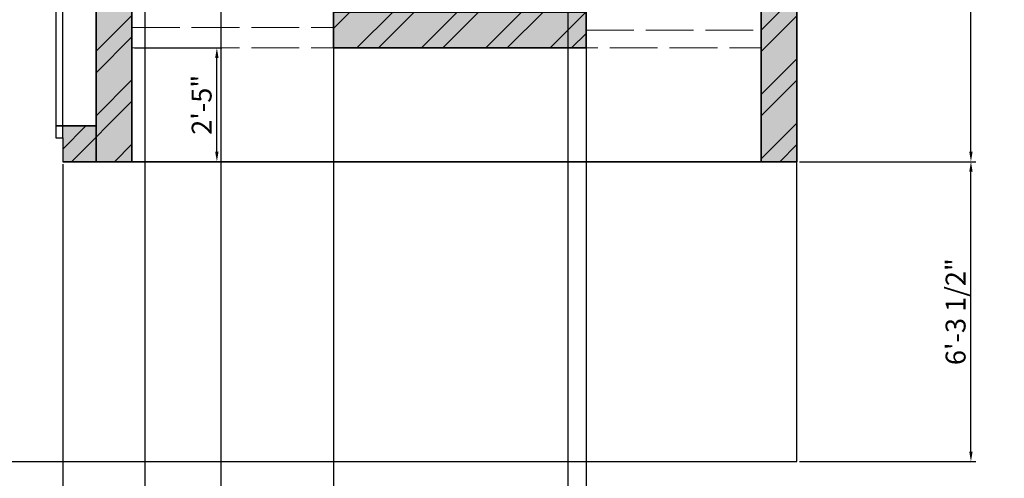
# Model space of a CAD drawing. Units: inches. Extents: x 1804 to 3296, y 909 to 2477.
# Tile 6 of 31: x 2130 to 2378, y 1059 to 1174. Entities that reach past the tile are written whole.
import ezdxf

# ---------------------------------------------------------------- set-up
doc = ezdxf.new("R2010")
doc.units = ezdxf.units.IN
doc.linetypes.add('ACAD_ISO02W100', pattern=[15, 12, -3])
for name, color, linetype, lineweight in [('A-ANNO-DIMS', 2, 'Continuous', 18), ('A-ANNO-TTLB', 156, 'Continuous', 35), ('A-GLAZ-OVHD', 130, 'ACAD_ISO02W100', 18), ('A-WALL-PATT', 10, 'Continuous', 13), ('C-PROP', 7, 'Continuous', 25), ('DOOR', 30, 'Continuous', 25), ('WALL', 10, 'Continuous', 35)]:
    doc.layers.add(name, color=color, linetype=linetype, lineweight=lineweight)
doc.styles.get("Standard").update_dxf_attribs({"font": 'arial.ttf'})
doc.dimstyles.new('ISO-25', dxfattribs={"dimtxt": 5, "dimasz": 2.5, "dimexe": 1.25, "dimexo": 0.625, "dimtad": 1, "dimdec": 0, "dimlunit": 4, "dimtxsty": 'Standard', "dimcen": 2.5, "dimadec": 0, "dimazin": 0, "dimtfac": 1, "dimtdec": 0, "dimtmove": 0, "dimatfit": 3, "dimfxl": 1, "dimarcsym": 0})

# ---------------------------------------------------------------- blocks, each defined once
blk = doc.blocks.new('*U2')
for p, q in [((0, 0), (0, -6)), ((40, 0), (40, -6))]:
    blk.add_line(p, q)
blk.add_lwpolyline([(0, 0), (0, 40), (1.75, 40), (1.75, 0)], close=True)
blk.add_arc((0, 0), 40, 0, 90)
blk = doc.blocks.new('*D20')
at = {"layer": 'A-ANNO-DIMS', "color": 0, "lineweight": -2, "transparency": 16777216}
for p, q in [((2159.2, 1166.63), (2181.16, 1166.63)), ((2179.91, 1140.57), (2179.91, 1164.13)), ((2159.2, 1138.07), (2181.16, 1138.07))]:
    blk.add_line(p, q, dxfattribs=at)
at = {"layer": 'A-ANNO-DIMS', "color": 0, "lineweight": 100, "transparency": 16777216}
for points in [[(2179.49, 1164.13), (2180.33, 1164.13), (2179.91, 1166.63)], [(2179.49, 1140.57), (2180.33, 1140.57), (2179.91, 1138.07)]]:
    blk.add_solid(points, dxfattribs=at)
at = {"layer": 'Defpoints', "color": 0, "lineweight": 100, "transparency": 16777216}
for p in [(2158.58, 1166.63), (2179.91, 1166.63), (2158.58, 1138.07)]:
    blk.add_point(p, dxfattribs=at)
at = {"layer": 'A-ANNO-DIMS', "color": 0, "transparency": 16777216, "insert": (2176.73, 1152.35), "char_height": 5, "attachment_point": 5, "rotation": 90}
blk.add_mtext('2\'-5"', dxfattribs=at)
blk = doc.blocks.new('*D22')
at = {"layer": 'A-ANNO-DIMS', "color": 0, "lineweight": -2, "transparency": 16777216}
for p, q in [((1934.58, 1147.69), (1934.58, 1206.88)), ((2149.58, 1147.69), (2149.58, 1206.88)), ((1937.08, 1205.63), (2147.08, 1205.63))]:
    blk.add_line(p, q, dxfattribs=at)
at = {"layer": 'A-ANNO-DIMS', "color": 0, "lineweight": 100, "transparency": 16777216}
for points in [[(1937.08, 1206.05), (1937.08, 1205.22), (1934.58, 1205.63)], [(2147.08, 1206.05), (2147.08, 1205.22), (2149.58, 1205.63)]]:
    blk.add_solid(points, dxfattribs=at)
at = {"layer": 'Defpoints', "color": 0, "lineweight": 100, "transparency": 16777216}
for p in [(2149.58, 1205.63), (1934.58, 1147.07), (2149.58, 1147.07)]:
    blk.add_point(p, dxfattribs=at)
at = {"layer": 'A-ANNO-DIMS', "color": 0, "transparency": 16777216, "insert": (2042.08, 1208.77), "char_height": 5, "attachment_point": 5}
blk.add_mtext('17\'-11"', dxfattribs=at)
blk = doc.blocks.new('*D53')
at = {"layer": 'A-ANNO-DIMS', "color": 0, "lineweight": -2, "transparency": 16777216}
for p, q in [((2326.16, 1793.38), (2370.49, 1793.38)), ((2369.24, 1140.57), (2369.24, 1790.88)), ((2326.16, 1138.07), (2370.49, 1138.07))]:
    blk.add_line(p, q, dxfattribs=at)
at = {"layer": 'A-ANNO-DIMS', "color": 0, "lineweight": 100, "transparency": 16777216}
for points in [[(2368.82, 1790.88), (2369.65, 1790.88), (2369.24, 1793.38)], [(2368.82, 1140.57), (2369.65, 1140.57), (2369.24, 1138.07)]]:
    blk.add_solid(points, dxfattribs=at)
at = {"layer": 'Defpoints', "color": 0, "lineweight": 100, "transparency": 16777216}
for p in [(2325.54, 1793.38), (2369.24, 1793.38), (2325.54, 1138.07)]:
    blk.add_point(p, dxfattribs=at)
at = {"layer": 'A-ANNO-DIMS', "color": 0, "transparency": 16777216, "insert": (2366.03, 1465.72), "char_height": 5, "attachment_point": 5, "rotation": 90}
blk.add_mtext('54\'-7 1/2"', dxfattribs=at)
blk = doc.blocks.new('*D54')
at = {"layer": 'A-ANNO-DIMS', "color": 0, "lineweight": -2, "transparency": 16777216}
for p, q in [((2326.16, 1138.07), (2370.49, 1138.07)), ((2369.24, 1065.27), (2369.24, 1135.57)), ((2326.16, 1062.77), (2370.49, 1062.77))]:
    blk.add_line(p, q, dxfattribs=at)
at = {"layer": 'A-ANNO-DIMS', "color": 0, "lineweight": 100, "transparency": 16777216}
for points in [[(2368.82, 1135.57), (2369.65, 1135.57), (2369.24, 1138.07)], [(2368.82, 1065.27), (2369.65, 1065.27), (2369.24, 1062.77)]]:
    blk.add_solid(points, dxfattribs=at)
at = {"layer": 'Defpoints', "color": 0, "lineweight": 100, "transparency": 16777216}
for p in [(2325.54, 1138.07), (2369.24, 1138.07), (2325.54, 1062.77)]:
    blk.add_point(p, dxfattribs=at)
at = {"layer": 'A-ANNO-DIMS', "color": 0, "transparency": 16777216, "insert": (2366.03, 1100.42), "char_height": 5, "attachment_point": 5, "rotation": 90}
blk.add_mtext('6\'-3 1/2"', dxfattribs=at)
blk = doc.blocks.new('*D56')
at = {"layer": 'A-ANNO-DIMS', "color": 0, "lineweight": -2, "transparency": 16777216}
for p, q in [((2180.87, 1680.42), (2180.87, 975.89)), ((2268, 1680.42), (2268, 975.89)), ((2183.37, 977.14), (2265.5, 977.14))]:
    blk.add_line(p, q, dxfattribs=at)
at = {"layer": 'A-ANNO-DIMS', "color": 0, "lineweight": 100, "transparency": 16777216}
for points in [[(2183.37, 977.56), (2183.37, 976.72), (2180.87, 977.14)], [(2265.5, 977.56), (2265.5, 976.72), (2268, 977.14)]]:
    blk.add_solid(points, dxfattribs=at)
at = {"layer": 'Defpoints', "color": 0, "lineweight": 100, "transparency": 16777216}
for p in [(2180.87, 1681.04), (2268, 1681.04), (2268, 977.14)]:
    blk.add_point(p, dxfattribs=at)
at = {"layer": 'A-ANNO-DIMS', "color": 0, "transparency": 16777216, "insert": (2224.44, 980.32), "char_height": 5, "attachment_point": 5}
blk.add_mtext('7\'-3"', dxfattribs=at)
blk = doc.blocks.new('*D59')
at = {"layer": 'A-ANNO-DIMS', "color": 0, "lineweight": -2, "transparency": 16777216}
for p, q in [((2121.83, 1590.3), (2121.83, 975.89)), ((2161.83, 1590.3), (2161.83, 975.89)), ((2124.33, 977.14), (2159.33, 977.14))]:
    blk.add_line(p, q, dxfattribs=at)
at = {"layer": 'A-ANNO-DIMS', "color": 0, "lineweight": 100, "transparency": 16777216}
for points in [[(2124.33, 977.56), (2124.33, 976.72), (2121.83, 977.14)], [(2159.33, 977.56), (2159.33, 976.72), (2161.83, 977.14)]]:
    blk.add_solid(points, dxfattribs=at)
at = {"layer": 'Defpoints', "color": 0, "lineweight": 100, "transparency": 16777216}
for p in [(2121.83, 1590.92), (2161.83, 1590.92), (2161.83, 977.14)]:
    blk.add_point(p, dxfattribs=at)
at = {"layer": 'A-ANNO-DIMS', "color": 0, "transparency": 16777216, "insert": (2141.83, 980.32), "char_height": 5, "attachment_point": 5}
blk.add_mtext('3\'-4"', dxfattribs=at)
blk = doc.blocks.new('*D61')
at = {"layer": 'A-ANNO-DIMS', "color": 0, "lineweight": -2, "transparency": 16777216}
for p, q in [((2101.21, 1137.44), (2101.21, 975.89)), ((2141.21, 1137.44), (2141.21, 975.89)), ((2103.71, 977.14), (2138.71, 977.14))]:
    blk.add_line(p, q, dxfattribs=at)
at = {"layer": 'A-ANNO-DIMS', "color": 0, "lineweight": 100, "transparency": 16777216}
for points in [[(2103.71, 977.56), (2103.71, 976.72), (2101.21, 977.14)], [(2138.71, 977.56), (2138.71, 976.72), (2141.21, 977.14)]]:
    blk.add_solid(points, dxfattribs=at)
at = {"layer": 'Defpoints', "color": 0, "lineweight": 100, "transparency": 16777216}
for p in [(2101.21, 1138.07), (2141.21, 1138.07), (2141.21, 977.14)]:
    blk.add_point(p, dxfattribs=at)
at = {"layer": 'A-ANNO-DIMS', "color": 0, "transparency": 16777216, "insert": (2121.21, 980.32), "char_height": 5, "attachment_point": 5}
blk.add_mtext('3\'-4"', dxfattribs=at)
blk = doc.blocks.new('*D69')
at = {"layer": 'A-ANNO-DIMS', "color": 0, "lineweight": -2, "transparency": 16777216}
for p, q in [((2209.19, 1223.01), (2209.19, 975.89)), ((2272.59, 1223.01), (2272.59, 975.89)), ((2211.69, 977.14), (2270.09, 977.14))]:
    blk.add_line(p, q, dxfattribs=at)
at = {"layer": 'A-ANNO-DIMS', "color": 0, "lineweight": 100, "transparency": 16777216}
for points in [[(2211.69, 977.56), (2211.69, 976.72), (2209.19, 977.14)], [(2270.09, 977.56), (2270.09, 976.72), (2272.59, 977.14)]]:
    blk.add_solid(points, dxfattribs=at)
at = {"layer": 'Defpoints', "color": 0, "lineweight": 100, "transparency": 16777216}
for p in [(2209.19, 1223.63), (2272.59, 1223.63), (2272.59, 977.14)]:
    blk.add_point(p, dxfattribs=at)
at = {"layer": 'A-ANNO-DIMS', "color": 0, "transparency": 16777216, "insert": (2240.89, 980.35), "char_height": 5, "attachment_point": 5}
blk.add_mtext('5\'-3 1/2"', dxfattribs=at)

msp = doc.modelspace()

# ---------------------------------------------------------------- hatches: boundary and pattern name
at = {"layer": 'A-ANNO-TTLB'}
h = msp.add_hatch(color=256, dxfattribs=at)
h.dxf.hatch_style = 1
h.paths.add_polyline_path([(3294.53, 2476.54), (1803.79, 2476.54), (1805.43, 909.47), (3296.17, 909.47)])
h.paths.add_polyline_path([(1811, 914.33), (1812.79, 2467.54), (3285.53, 2467.54), (3283.74, 914.33)], flags=16)
h.paths.add_polyline_path([(1925.58, 1062.77), (1925.58, 1138.07), (1925.58, 1539.88), (1925.58, 1793.38), (1925.58, 1830.04), (2325.54, 1830.04), (2325.54, 1793.38), (2325.54, 1586.42), (2325.54, 1138.07), (2325.54, 1062.77)], flags=0)
h.paths.add_polyline_path([(1997.22, 1029.4), (2008.85, 1037.96), (2008.85, 1020.84)], flags=0)
h.paths.add_polyline_path([(1934.58, 1138.07), (1934.58, 1147.07), (2078.77, 1147.07), (2078.77, 1138.07), (2060.94, 1138.07)], flags=0)
h.paths.add_polyline_path([(1944.35, 1138.07), (1944.35, 1147.07), (2056.05, 1147.07), (2056.05, 1138.07)], flags=0)
h.paths.add_polyline_path([(2222.24, 1037.96), (2233.87, 1029.4), (2222.24, 1020.84)], flags=0)
h.paths.add_polyline_path([(2061.94, 1139.07), (2061.94, 1146.07), (2077.77, 1146.07), (2077.77, 1139.07)], flags=0)
h.paths.add_polyline_path([(2149.58, 1138.07), (2149.58, 1269.44), (2158.58, 1269.44), (2158.58, 1326.69), (2149.58, 1326.69), (2149.58, 1340.94), (2139.6, 1340.94), (2139.6, 1434.25), (2149.58, 1434.25), (2149.58, 1447.36), (2158.58, 1447.36), (2158.58, 1423.87), (2158.58, 1408.06), (2198.46, 1408.06), (2198.46, 1412.56), (2282.65, 1412.56), (2282.65, 1465.94), (2316.54, 1465.94), (2316.54, 1590.92), (2192.86, 1590.92), (2192.86, 1595.3), (2291.17, 1595.3), (2291.17, 1590.92), (2316.54, 1590.92), (2316.54, 1784.38), (2300.24, 1784.38), (2300.24, 1757.47), (2268, 1757.47), (2268, 1681.04), (2180.87, 1681.04), (2180.87, 1757.47), (2148.63, 1757.47), (2148.63, 1784.38), (2119.08, 1784.38), (2119.08, 1585.58), (2114.58, 1585.58), (2114.58, 1784.38), (2064.11, 1784.38), (2046.28, 1784.38), (2046.28, 1760.38), (1958.58, 1760.38), (1958.58, 1664.38), (1934.58, 1664.38), (1934.58, 1784.38), (1934.58, 1793.38), (2046.28, 1793.38), (2064.11, 1793.38), (2119.08, 1793.38), (2230.78, 1793.38), (2230.78, 1784.38), (2268, 1784.38), (2300.24, 1784.38), (2316.54, 1784.38), (2316.54, 1590.92), (2316.54, 1373.73), (2316.54, 1138.07)], flags=0)
h.paths.add_polyline_path([(2209.19, 1166.63), (2209.19, 1175.63), (2158.58, 1175.63), (2209.19, 1223.63), (2209.19, 1231.63), (2183.88, 1231.63), (2183.88, 1301.66), (2242.59, 1301.66), (2242.59, 1326.69), (2316.54, 1326.69), (2272.59, 1271.63), (2272.59, 1223.63), (2316.54, 1175.63), (2272.59, 1175.63), (2272.59, 1166.63)], flags=0)
h.paths.add_polyline_path([(1947.77, 1345.22), (1947.77, 1457.48), (1991.2, 1457.48), (1991.2, 1451.7), (1991.2, 1352.18), (1991.2, 1345.22)], flags=0)
h.paths.add_polyline_path([(2209.19, 1271.63), (2262.59, 1271.63), (2262.59, 1311.85), (2272.59, 1301.66), (2272.59, 1271.63), (2269.92, 1269.63), (2270.59, 1269.63), (2270.59, 1225.63), (2211.19, 1225.63), (2211.19, 1269.63), (2211.86, 1269.63)], flags=0)
h.paths.add_polyline_path([(2000.34, 1378.21), (2000.34, 1429.71), (2025.22, 1429.71), (2025.22, 1378.21)], flags=0)
h.paths.add_polyline_path([(2001.34, 1379.21), (2001.34, 1428.71), (2024.22, 1428.71), (2024.22, 1379.21)], flags=0)
h.paths.add_polyline_path([(2012.34, 1390.21), (2012.34, 1417.71), (2013.22, 1417.71), (2013.22, 1390.21)], flags=0)
h.paths.add_polyline_path([(2237.56, 1331.19), (2237.56, 1340.18), (2238.62, 1340.18), (2238.62, 1386.84), (2241.04, 1386.84), (2242.06, 1386.84), (2242.06, 1408.06), (2316.54, 1331.19)], flags=0)
h.paths.add_polyline_path([(1953.73, 1464.35), (1953.73, 1498.59), (1981.74, 1498.59), (1981.74, 1464.35)], flags=0)
h.paths.add_polyline_path([(1987.63, 1462.08), (1987.63, 1500.95), (2104.07, 1500.95), (2104.07, 1462.08), (2099.27, 1462.08), (1993.6, 1462.08)], flags=0)
h.paths.add_polyline_path([(1956.06, 1481.47, -1), (1979.41, 1481.47, -1)], flags=0)
edge = h.paths.add_edge_path(flags=0)
edge.add_ellipse((2299.53, 1438.37), major_axis=(0.31, 21.36), ratio=0.670333, start_angle=0, end_angle=360)
h.paths.add_polyline_path([(2297.39, 1438.37, -1), (2301.67, 1438.37, -1)], flags=0)
h.paths.add_polyline_path([(2591.54, 1163.23), (2591.54, 1179.38), (2591.54, 1379.68), (2591.54, 1395.84), (2734.5, 1395.84), (2734.5, 1379.68), (2734.5, 1179.38), (2734.5, 1163.23)], flags=0)
h.paths.add_polyline_path([(2592.54, 1164.23), (2592.54, 1166.23), (2733.5, 1166.23), (2733.5, 1164.23)], flags=0)
h.paths.add_polyline_path([(2592.54, 1180.38), (2592.54, 1378.68), (2733.5, 1378.68), (2733.5, 1180.38)], flags=0)
h.paths.add_polyline_path([(2593.54, 1181.38), (2593.54, 1377.68), (2732.5, 1377.68), (2732.5, 1181.38)], flags=0)
h.paths.add_polyline_path([(2594.54, 1182.38), (2594.54, 1376.68), (2731.5, 1376.68), (2731.5, 1182.38)], flags=0)
h.paths.add_polyline_path([(1936.95, 1697.46), (1936.95, 1736.46), (1955.41, 1736.46), (1955.41, 1697.46)], flags=0)
h.paths.add_polyline_path([(1938.48, 1718.36), (1938.48, 1734.92), (1953.65, 1734.92), (1953.65, 1718.36)], flags=0)
h.paths.add_polyline_path([(1944.75, 1726.64, -1), (1947.37, 1726.64, -1)], flags=0)
h.paths.add_polyline_path([(2592.54, 1394.84), (2733.5, 1394.84), (2733.5, 1392.84), (2592.54, 1392.84)], flags=0)
h.paths.add_polyline_path([(1976.61, 1762.5), (1976.61, 1781.44), (2012.79, 1781.44), (2012.79, 1762.5)], flags=0)
h.paths.add_polyline_path([(1979.57, 1771.97, -1), (1991.39, 1771.97, -1)], flags=0)
h.paths.add_polyline_path([(1995.36, 1771.97, -1), (2007.18, 1771.97, -1)], flags=0)
h.paths.add_polyline_path([(2251.51, 1744.53), (2268, 1730.05), (2251.51, 1730.05)], flags=0)
h.paths.add_polyline_path([(2047.28, 1785.38), (2047.28, 1792.38), (2063.11, 1792.38), (2063.11, 1785.38)], flags=0)
h.paths.add_polyline_path([(2155.08, 1770.92, -1), (2174.42, 1770.92, -1)], flags=0)
h.paths.add_polyline_path([(2188.59, 1758.27), (2188.59, 1772.81), (2222.3, 1772.81), (2222.3, 1758.27)], flags=0)
h.paths.add_polyline_path([(2223.97, 1758.27), (2223.97, 1772.81), (2257.68, 1772.81), (2257.68, 1758.27)], flags=0)
h.paths.add_polyline_path([(2274.45, 1770.92, -1), (2293.8, 1770.92, -1)], flags=0)
h.paths.add_polyline_path([(2591.54, 1582.09), (2591.54, 1782.39), (2734.5, 1782.39), (2734.5, 1582.09)], flags=0)
h.paths.add_polyline_path([(2592.54, 1583.09), (2592.54, 1781.39), (2733.5, 1781.39), (2733.5, 1583.09)], flags=0)
h.paths.add_polyline_path([(2593.54, 1584.09), (2593.54, 1780.39), (2732.5, 1780.39), (2732.5, 1584.09)], flags=0)
h.paths.add_polyline_path([(2594.54, 1585.09), (2594.54, 1779.39), (2731.5, 1779.39), (2731.5, 1585.09)], flags=0)
h.paths.add_polyline_path([(1922.17, 1978.79), (1922.17, 2295.08), (1922.17, 2296.08), (2115.67, 2296.08), (2115.67, 2384.31), (2115.67, 2385.31), (2322.12, 2385.31), (2323.12, 2385.31), (2323.12, 1979.79), (2323.12, 1978.79), (1923.17, 1978.79)], flags=0)
h.paths.add_polyline_path([(1922.17, 1978.79), (1922.17, 2051.31), (1922.17, 2214.86), (1922.17, 2296.08), (2115.67, 2296.08), (2115.67, 2385.31), (2323.12, 2385.31), (2323.12, 2280.42), (2323.12, 1978.79), (2115.67, 1978.79)], flags=0)
h.paths.add_polyline_path([(1923.17, 1979.79), (1923.17, 2050.31), (2115.67, 2050.31), (2115.67, 2051.31), (1923.17, 2051.31), (1923.17, 2213.86), (1923.17, 2214.86), (1923.17, 2295.08), (1990.02, 2295.08), (1990.02, 2214.86), (1991.02, 2214.86), (1991.02, 2295.08), (2115.67, 2295.08), (2115.67, 1979.79), (2116.67, 1979.79), (2116.67, 2304.18), (2116.67, 2384.31), (2322.12, 2384.31), (2322.12, 2280.42), (2322.12, 1979.79), (2115.67, 1979.79)], flags=0)
h.paths.add_polyline_path([(2972.46, 1192.5), (2972.46, 1196.92), (2995.47, 1196.92), (2995.47, 1255.47), (2995.09, 1255.47), (2987.42, 1249.39), (2980.08, 1255.47), (2978.05, 1255.47), (2978.05, 1257.24), (2995.47, 1257.24), (2995.47, 1261.58), (3015.37, 1261.58), (3015.37, 1333.28), (3015.37, 1414.4), (3032.82, 1414.4), (3032.82, 1333.28), (3032.82, 1261.58), (3052.66, 1261.58), (3052.66, 1255.47), (3079.86, 1255.47), (3078.72, 1254.57), (3081.47, 1252.29), (3078.56, 1249.99), (3075.81, 1252.26), (3072.57, 1249.69), (3070.36, 1251.52), (3067.67, 1249.39), (3060.34, 1255.47), (3052.66, 1255.47), (3052.66, 1196.92), (3054.58, 1196.92), (3074, 1196.92), (3074, 1192.5), (3052.66, 1192.5), (2995.47, 1192.5)], flags=0)
h.paths.add_polyline_path([(2490.75, 1979.27), (2490.75, 1980.27), (2596.87, 1980.27), (2596.87, 2051.8), (2596.87, 2052.8), (2596.87, 2216.35), (2596.87, 2297.57), (2717.32, 2297.57), (2710.57, 2305.62), (2724.07, 2305.62), (2717.32, 2297.57), (2782.37, 2297.57), (2782.37, 2395.8), (3006.82, 2395.8), (3006.82, 1981.27), (3093.73, 1981.27), (3093.73, 1980.27), (3047.51, 1980.27), (3046.37, 1979.37), (3049.11, 1977.1), (3046.2, 1974.79), (3043.46, 1977.07), (3040.21, 1974.49), (3038, 1976.32), (3035.32, 1974.2), (3027.98, 1980.27), (2871.83, 1980.27), (2871.83, 1981.27), (2791.37, 1981.27), (2791.37, 2050.8), (2597.87, 2050.8), (2597.87, 1980.27), (2597.87, 1979.27), (2546.27, 1979.27), (2545.12, 1978.37), (2547.87, 1976.1), (2544.96, 1973.79), (2542.22, 1976.07), (2538.97, 1973.49), (2536.76, 1975.32), (2534.07, 1973.2), (2526.74, 1979.27)], flags=0)
h.paths.add_polyline_path([(2597.87, 2051.8), (2606.87, 2051.8), (2606.87, 2258.39), (2597.87, 2258.39), (2597.87, 2296.57), (2606.87, 2296.57), (2606.87, 2262.39), (2782.37, 2262.39), (2782.37, 2296.57), (2790.37, 2296.57), (2790.37, 2262.39), (2791.37, 2262.39), (2791.37, 2305.67), (2791.37, 2385.8), (2996.82, 2385.8), (2996.82, 2339.85), (3006.82, 2339.85), (3006.82, 2250.12), (2997.82, 2250.12), (2997.82, 1981.27), (2996.82, 1981.27), (2872.83, 1981.27), (2872.83, 1991.8), (2871.83, 1991.8), (2871.83, 2050.8), (2790.37, 2050.8), (2597.87, 2050.8)], flags=0)
h.paths.add_polyline_path([(2179.93, 2153.92), (2179.93, 2353.97), (2259.98, 2353.97), (2259.98, 2153.92)], flags=0)
h.paths.add_polyline_path([(2180.93, 2154.92), (2180.93, 2352.97), (2258.98, 2352.97), (2258.98, 2154.92)], flags=0)
h.paths.add_polyline_path([(2960.87, 1608.49), (2960.87, 1753.62), (3070.9, 1753.62), (3070.9, 1608.49)], flags=0)
h.paths.add_polyline_path([(2961.87, 1609.49), (2961.87, 1752.62), (3069.9, 1752.62), (3069.9, 1609.49)], flags=0)
h.paths.add_polyline_path([(2962.87, 1610.49), (2962.87, 1751.62), (3068.9, 1751.62), (3068.9, 1610.49)], flags=0)
h.paths.add_polyline_path([(2963.87, 1611.49), (2963.87, 1750.62), (3067.9, 1750.62), (3067.9, 1611.49)], flags=0)
h.paths.add_polyline_path([(2782.37, 2051.8), (2782.37, 2216.32), (2791.37, 2216.32), (2791.37, 2051.8), (2872.83, 2051.8), (2872.83, 2068.56), (2884.67, 2068.56), (2884.67, 2085.33), (2896.51, 2085.33), (2896.51, 2102.09), (2908.36, 2102.09), (2908.36, 2118.85), (2920.2, 2118.85), (2920.2, 2135.62), (2932.05, 2135.62), (2932.05, 2145.3), (2925.08, 2145.3), (2925.08, 2203.2), (2996.82, 2203.2), (2996.82, 2145.3), (2953.82, 2145.3), (2872.83, 2051.8), (2790.37, 2051.8)], flags=0)
h.paths.add_polyline_path([(2717.32, 2238.65), (2710.57, 2246.7), (2724.07, 2246.7)], flags=0)
h.paths.add_polyline_path([(2003.09, 1122.79), (2017.16, 1122.79), (2017.16, 1138.74), (2003.09, 1138.74)], flags=8)
h.paths.add_polyline_path([(2174.76, 1792.72), (2188.83, 1792.72), (2188.83, 1808.66), (2174.76, 1808.66)], flags=8)
h.paths.add_polyline_path([(1987.95, 1792.51), (2002.02, 1792.51), (2002.02, 1808.45), (1987.95, 1808.45)], flags=8)
h.paths.add_polyline_path([(2148.79, 1289.26), (2160.46, 1289.26), (2160.46, 1305.2), (2148.79, 1305.2)], flags=8)
h.paths.add_polyline_path([(2115.36, 1133.57), (2127.04, 1133.57), (2127.04, 1149.51), (2115.36, 1149.51)], flags=8)
h.paths.add_polyline_path([(2237.58, 1421.48), (2249.25, 1421.48), (2249.25, 1437.43), (2237.58, 1437.43)], flags=8)
h.paths.add_polyline_path([(2134.99, 1584.32), (2146.66, 1584.32), (2146.66, 1600.26), (2134.99, 1600.26)], flags=8)
h.paths.add_polyline_path([(2101.95, 1557.31), (2113.62, 1557.31), (2113.62, 1573.25), (2101.95, 1573.25)], flags=8)
h.paths.add_polyline_path([(2937.85, 1156.77), (3120.41, 1156.77), (3120.41, 1185.72), (2937.85, 1185.72)], flags=8)
h.paths.add_polyline_path([(2980.71, 1786.71), (3050.06, 1786.71), (3050.06, 1802.66), (2980.71, 1802.66)], flags=8)
h.paths.add_polyline_path([(2869.28, 1661.96), (2938.62, 1661.96), (2938.62, 1690.8), (2869.28, 1690.8)], flags=8)
h.paths.add_polyline_path([(3092.27, 1674.86), (3161.62, 1674.86), (3161.62, 1690.8), (3092.27, 1690.8)], flags=8)
h.paths.add_polyline_path([(2980.71, 1674.86), (3050.06, 1674.86), (3050.06, 1690.8), (2980.71, 1690.8)], flags=8)
h.paths.add_polyline_path([(2649.07, 1678.23), (2674.53, 1678.23), (2674.53, 1714.76), (2649.07, 1714.76)], flags=8)
h.paths.add_polyline_path([(2530.84, 1981.63), (2549.13, 1981.63), (2549.13, 1997.57), (2530.84, 1997.57)], flags=8)
h.paths.add_polyline_path([(3031.29, 1981.77), (3049.58, 1981.77), (3049.58, 1997.71), (3031.29, 1997.71)], flags=8)
h.paths.add_polyline_path([(2715.38, 1911.9), (2851.54, 1911.9), (2851.54, 1940.85), (2715.38, 1940.85)], flags=8)
h.paths.add_polyline_path([(2015.23, 1927.36), (2205.42, 1927.36), (2205.42, 1956.3), (2015.23, 1956.3)], flags=8)
h.paths.add_polyline_path([(2671.84, 2057.84), (2702.75, 2057.84), (2702.75, 2073.79), (2671.84, 2073.79)], flags=8)
h.paths.add_polyline_path([(2678.5, 2316.52), (2765.26, 2316.52), (2765.26, 2332.46), (2678.5, 2332.46)], flags=8)
h.paths.add_polyline_path([(2678.48, 2271.96), (2736.41, 2271.96), (2736.41, 2287.9), (2678.48, 2287.9)], flags=8)
h.paths.add_polyline_path([(2019.2, 972.79), (2243.21, 972.79), (2243.21, 1001.74), (2019.2, 1001.74)], flags=8)
h.paths.add_polyline_path([(2097.06, 1021.56), (2132.16, 1021.56), (2132.16, 1037.51), (2097.06, 1037.51)], flags=8)
h.paths.add_polyline_path([(2182.47, 1360.48), (2207.35, 1360.48), (2207.35, 1376.42), (2182.47, 1376.42)], flags=8)
h.paths.add_polyline_path([(2261.12, 1361.77), (2295.01, 1361.77), (2295.01, 1377.71), (2261.12, 1377.71)], flags=8)
h.paths.add_polyline_path([(2245.75, 1511.51), (2278.44, 1511.51), (2278.44, 1527.46), (2245.75, 1527.46)], flags=8)
h.paths.add_polyline_path([(1991.16, 1296.29), (2060.51, 1296.29), (2060.51, 1312.23), (1991.16, 1312.23)], flags=8)
h.paths.add_polyline_path([(2187, 1651.35), (2246.71, 1651.35), (2246.71, 1667.29), (2187, 1667.29)], flags=8)
h.paths.add_polyline_path([(1976.49, 1684.81), (2068.63, 1684.81), (2068.63, 1700.76), (1976.49, 1700.76)], flags=8)
at = {"layer": 'A-WALL-PATT'}
h = msp.add_hatch(color=256, dxfattribs=at)
h.dxf.hatch_style = 1
h.paths.add_polyline_path([(2149.58, 1147.07), (2141.21, 1147.07), (2141.21, 1144.07), (2141.21, 1138.07), (2149.58, 1138.07)])
h.paths.add_polyline_path([(2101.21, 1144.07, -0.01877), (2101.32, 1147.07), (2078.77, 1147.07), (2078.77, 1138.07), (2101.21, 1138.07)])
h.paths.add_polyline_path([(2060.94, 1147.07), (2056.05, 1147.07), (2056.05, 1138.07), (2060.94, 1138.07)])
h.paths.add_polyline_path([(1944.35, 1147.07), (1934.58, 1147.07), (1934.58, 1138.07), (1944.35, 1138.07)])
h.paths.add_polyline_path([(2158.58, 1269.44), (2149.58, 1269.44), (2149.58, 1138.07), (2158.58, 1138.07)])
h.paths.add_polyline_path([(2003.09, 1122.79), (2017.16, 1122.79), (2017.16, 1138.74), (2003.09, 1138.74)], flags=9)
h.paths.add_polyline_path([(2174.76, 1792.72), (2188.83, 1792.72), (2188.83, 1808.66), (2174.76, 1808.66)], flags=9)
h.paths.add_polyline_path([(1987.95, 1792.51), (2002.02, 1792.51), (2002.02, 1808.45), (1987.95, 1808.45)], flags=9)
h.paths.add_polyline_path([(2148.79, 1289.26), (2160.46, 1289.26), (2160.46, 1305.2), (2148.79, 1305.2)], flags=9)
h.paths.add_polyline_path([(2115.36, 1133.57), (2127.04, 1133.57), (2127.04, 1149.51), (2115.36, 1149.51)], flags=9)
h.paths.add_polyline_path([(2237.58, 1421.48), (2249.25, 1421.48), (2249.25, 1437.43), (2237.58, 1437.43)], flags=9)
h.paths.add_polyline_path([(2134.99, 1584.32), (2146.66, 1584.32), (2146.66, 1600.26), (2134.99, 1600.26)], flags=9)
h.paths.add_polyline_path([(2101.95, 1557.31), (2113.62, 1557.31), (2113.62, 1573.25), (2101.95, 1573.25)], flags=9)
h.paths.add_polyline_path([(2937.85, 1156.77), (3120.41, 1156.77), (3120.41, 1185.72), (2937.85, 1185.72)], flags=9)
h.paths.add_polyline_path([(2980.71, 1786.71), (3050.06, 1786.71), (3050.06, 1802.66), (2980.71, 1802.66)], flags=9)
h.paths.add_polyline_path([(2869.28, 1661.96), (2938.62, 1661.96), (2938.62, 1690.8), (2869.28, 1690.8)], flags=9)
h.paths.add_polyline_path([(3092.27, 1674.86), (3161.62, 1674.86), (3161.62, 1690.8), (3092.27, 1690.8)], flags=9)
h.paths.add_polyline_path([(2980.71, 1674.86), (3050.06, 1674.86), (3050.06, 1690.8), (2980.71, 1690.8)], flags=9)
h.paths.add_polyline_path([(2649.07, 1678.23), (2674.53, 1678.23), (2674.53, 1714.76), (2649.07, 1714.76)], flags=9)
h.paths.add_polyline_path([(2530.84, 1981.63), (2549.13, 1981.63), (2549.13, 1997.57), (2530.84, 1997.57)], flags=9)
h.paths.add_polyline_path([(3031.29, 1981.77), (3049.58, 1981.77), (3049.58, 1997.71), (3031.29, 1997.71)], flags=9)
h.paths.add_polyline_path([(2715.38, 1911.9), (2851.54, 1911.9), (2851.54, 1940.85), (2715.38, 1940.85)], flags=9)
h.paths.add_polyline_path([(2015.23, 1927.36), (2205.42, 1927.36), (2205.42, 1956.3), (2015.23, 1956.3)], flags=9)
h.paths.add_polyline_path([(2671.84, 2057.84), (2702.75, 2057.84), (2702.75, 2073.79), (2671.84, 2073.79)], flags=9)
h.paths.add_polyline_path([(2678.5, 2316.52), (2765.26, 2316.52), (2765.26, 2332.46), (2678.5, 2332.46)], flags=9)
h.paths.add_polyline_path([(2678.48, 2271.96), (2736.41, 2271.96), (2736.41, 2287.9), (2678.48, 2287.9)], flags=9)
h.paths.add_polyline_path([(2019.2, 972.79), (2243.21, 972.79), (2243.21, 1001.74), (2019.2, 1001.74)], flags=9)
h.paths.add_polyline_path([(2097.06, 1021.56), (2132.16, 1021.56), (2132.16, 1037.51), (2097.06, 1037.51)], flags=9)
h.paths.add_polyline_path([(2182.47, 1360.48), (2207.35, 1360.48), (2207.35, 1376.42), (2182.47, 1376.42)], flags=9)
h.paths.add_polyline_path([(2261.12, 1361.77), (2295.01, 1361.77), (2295.01, 1377.71), (2261.12, 1377.71)], flags=9)
h.paths.add_polyline_path([(2245.75, 1511.51), (2278.44, 1511.51), (2278.44, 1527.46), (2245.75, 1527.46)], flags=9)
h.paths.add_polyline_path([(1991.16, 1296.29), (2060.51, 1296.29), (2060.51, 1312.23), (1991.16, 1312.23)], flags=9)
h.paths.add_polyline_path([(2187, 1651.35), (2246.71, 1651.35), (2246.71, 1667.29), (2187, 1667.29)], flags=9)
h.paths.add_polyline_path([(1976.49, 1684.81), (2068.63, 1684.81), (2068.63, 1700.76), (1976.49, 1700.76)], flags=9)
h = msp.add_hatch(color=256, dxfattribs=at)
h.dxf.hatch_style = 1
h.paths.add_polyline_path([(2158.58, 1275.49), (2155.29, 1275.49), (2149.58, 1275.49), (2149.58, 1269.44), (2158.58, 1269.44)])
h.paths.add_polyline_path([(2158.58, 1326.69), (2149.58, 1326.69), (2149.58, 1319.33), (2155.29, 1319.33), (2158.58, 1319.33)])
h.paths.add_polyline_path([(2158.58, 1402.2), (2158.58, 1423.87), (2158.58, 1447.36), (2149.58, 1447.36), (2149.58, 1423.87), (2149.58, 1340.94), (2149.58, 1326.69), (2158.58, 1326.69), (2158.58, 1354.23)])
h.paths.add_polyline_path([(1965.87, 1658.79), (1965.87, 1679.09), (1955.57, 1679.09), (1955.57, 1658.79)], flags=9)
h.paths.add_polyline_path([(2293.18, 1677.29), (2293.18, 1697.58), (2282.88, 1697.58), (2282.88, 1677.29)], flags=9)
h.paths.add_polyline_path([(2271.13, 1545.23), (2287.53, 1545.23), (2287.53, 1555.53), (2271.13, 1555.53)], flags=9)
h.paths.add_polyline_path([(2303.26, 1488.52), (2303.26, 1508.82), (2292.95, 1508.82), (2292.95, 1488.52)], flags=9)
h.paths.add_polyline_path([(2271.13, 1393.15), (2287.53, 1393.15), (2287.53, 1403.45), (2271.13, 1403.45)], flags=9)
h.paths.add_polyline_path([(2306.48, 1361.45), (2306.48, 1377.86), (2296.18, 1377.86), (2296.18, 1361.45)], flags=9)
h.paths.add_polyline_path([(2189.9, 1340.62), (2206.31, 1340.62), (2206.31, 1350.92), (2189.9, 1350.92)], flags=9)
h.paths.add_polyline_path([(2174.54, 1361.45), (2174.54, 1377.86), (2164.23, 1377.86), (2164.23, 1361.45)], flags=9)
h.paths.add_polyline_path([(2304.24, 1240.8), (2304.24, 1261.09), (2293.94, 1261.09), (2293.94, 1240.8)], flags=9)
h.paths.add_polyline_path([(2227.19, 1188.73), (2247.49, 1188.73), (2247.49, 1199.03), (2227.19, 1199.03)], flags=9)
h.paths.add_polyline_path([(2181.93, 1144.21), (2181.93, 1160.62), (2171.63, 1160.62), (2171.63, 1144.21)], flags=9)
h.paths.add_polyline_path([(1968.21, 1333.34), (1968.21, 1353.64), (1957.91, 1353.64), (1957.91, 1333.34)], flags=9)
h.paths.add_polyline_path([(2029.78, 1203.53), (2053.95, 1203.53), (2053.95, 1213.83), (2029.78, 1213.83)], flags=9)
h.paths.add_polyline_path([(2576.51, 1671.88), (2576.51, 1692.17), (2566.21, 1692.17), (2566.21, 1671.88)], flags=9)
h.paths.add_polyline_path([(2566.99, 1269.67), (2566.99, 1289.96), (2556.68, 1289.96), (2556.68, 1269.67)], flags=9)
h.paths.add_polyline_path([(2581.85, 1269.17), (2581.85, 1289.46), (2571.54, 1289.46), (2571.54, 1269.17)], flags=9)
h.paths.add_polyline_path([(2650.71, 1409.75), (2674.89, 1409.75), (2674.89, 1420.05), (2650.71, 1420.05)], flags=9)
h.paths.add_polyline_path([(2003.09, 1122.79), (2017.16, 1122.79), (2017.16, 1138.74), (2003.09, 1138.74)], flags=9)
h.paths.add_polyline_path([(2174.76, 1792.72), (2188.83, 1792.72), (2188.83, 1808.66), (2174.76, 1808.66)], flags=9)
h.paths.add_polyline_path([(1987.95, 1792.51), (2002.02, 1792.51), (2002.02, 1808.45), (1987.95, 1808.45)], flags=9)
h.paths.add_polyline_path([(2148.79, 1289.26), (2160.46, 1289.26), (2160.46, 1305.2), (2148.79, 1305.2)], flags=9)
h.paths.add_polyline_path([(2115.36, 1133.57), (2127.04, 1133.57), (2127.04, 1149.51), (2115.36, 1149.51)], flags=9)
h.paths.add_polyline_path([(2237.58, 1421.48), (2249.25, 1421.48), (2249.25, 1437.43), (2237.58, 1437.43)], flags=9)
h.paths.add_polyline_path([(2134.99, 1584.32), (2146.66, 1584.32), (2146.66, 1600.26), (2134.99, 1600.26)], flags=9)
h.paths.add_polyline_path([(2101.95, 1557.31), (2113.62, 1557.31), (2113.62, 1573.25), (2101.95, 1573.25)], flags=9)
h.paths.add_polyline_path([(2937.85, 1156.77), (3120.41, 1156.77), (3120.41, 1185.72), (2937.85, 1185.72)], flags=9)
h.paths.add_polyline_path([(2980.71, 1786.71), (3050.06, 1786.71), (3050.06, 1802.66), (2980.71, 1802.66)], flags=9)
h.paths.add_polyline_path([(2869.28, 1661.96), (2938.62, 1661.96), (2938.62, 1690.8), (2869.28, 1690.8)], flags=9)
h.paths.add_polyline_path([(3092.27, 1674.86), (3161.62, 1674.86), (3161.62, 1690.8), (3092.27, 1690.8)], flags=9)
h.paths.add_polyline_path([(2980.71, 1674.86), (3050.06, 1674.86), (3050.06, 1690.8), (2980.71, 1690.8)], flags=9)
h.paths.add_polyline_path([(2649.07, 1678.23), (2674.53, 1678.23), (2674.53, 1714.76), (2649.07, 1714.76)], flags=9)
h.paths.add_polyline_path([(2530.84, 1981.63), (2549.13, 1981.63), (2549.13, 1997.57), (2530.84, 1997.57)], flags=9)
h.paths.add_polyline_path([(3031.29, 1981.77), (3049.58, 1981.77), (3049.58, 1997.71), (3031.29, 1997.71)], flags=9)
h.paths.add_polyline_path([(2715.38, 1911.9), (2851.54, 1911.9), (2851.54, 1940.85), (2715.38, 1940.85)], flags=9)
h.paths.add_polyline_path([(2015.23, 1927.36), (2205.42, 1927.36), (2205.42, 1956.3), (2015.23, 1956.3)], flags=9)
h.paths.add_polyline_path([(2671.84, 2057.84), (2702.75, 2057.84), (2702.75, 2073.79), (2671.84, 2073.79)], flags=9)
h.paths.add_polyline_path([(2678.5, 2316.52), (2765.26, 2316.52), (2765.26, 2332.46), (2678.5, 2332.46)], flags=9)
h.paths.add_polyline_path([(2678.48, 2271.96), (2736.41, 2271.96), (2736.41, 2287.9), (2678.48, 2287.9)], flags=9)
h.paths.add_polyline_path([(2019.2, 972.79), (2243.21, 972.79), (2243.21, 1001.74), (2019.2, 1001.74)], flags=9)
h.paths.add_polyline_path([(2097.06, 1021.56), (2132.16, 1021.56), (2132.16, 1037.51), (2097.06, 1037.51)], flags=9)
h.paths.add_polyline_path([(2182.47, 1360.48), (2207.35, 1360.48), (2207.35, 1376.42), (2182.47, 1376.42)], flags=9)
h.paths.add_polyline_path([(2261.12, 1361.77), (2295.01, 1361.77), (2295.01, 1377.71), (2261.12, 1377.71)], flags=9)
h.paths.add_polyline_path([(2245.75, 1511.51), (2278.44, 1511.51), (2278.44, 1527.46), (2245.75, 1527.46)], flags=9)
h.paths.add_polyline_path([(1991.16, 1296.29), (2060.51, 1296.29), (2060.51, 1312.23), (1991.16, 1312.23)], flags=9)
h.paths.add_polyline_path([(2187, 1651.35), (2246.71, 1651.35), (2246.71, 1667.29), (2187, 1667.29)], flags=9)
h.paths.add_polyline_path([(1976.49, 1684.81), (2068.63, 1684.81), (2068.63, 1700.76), (1976.49, 1700.76)], flags=9)
h = msp.add_hatch(dxfattribs=at)
h.set_pattern_fill('ANSI32', color=256, scale=1.2)
h.set_pattern_definition([(45, (0, 196.207), (-8.08223, 8.08223), []), (45, (5.388, 196.207), (-8.08223, 8.08223), [])])
h.paths.add_polyline_path([(1934.58, 1784.38), (1934.58, 1793.38), (1925.58, 1793.38), (1925.58, 1539.88), (2119.08, 1539.88), (2119.08, 1545.58), (2114.58, 1545.58), (2114.58, 1544.38), (1934.58, 1544.38)])
h.paths.add_polyline_path([(2114.58, 1793.38), (2064.11, 1793.38), (2064.11, 1784.38), (2114.58, 1784.38)], flags=17)
h.paths.add_polyline_path([(2325.54, 1793.38), (2230.78, 1793.38), (2230.78, 1784.38), (2268, 1784.38), (2300.24, 1784.38), (2316.54, 1784.38), (2316.54, 1590.92), (2316.54, 1586.42), (2325.54, 1586.42)])
h.paths.add_polyline_path([(1944.35, 1147.07), (1934.58, 1147.07), (1934.58, 1138.07), (1944.35, 1138.07)])
h.paths.add_polyline_path([(2101.21, 1144.07, -0.01877), (2101.32, 1147.07), (2078.77, 1147.07), (2078.77, 1138.07), (2101.21, 1138.07)])
h.paths.add_polyline_path([(1934.58, 1539.88), (1925.58, 1539.88), (1925.58, 1138.07), (1934.58, 1138.07), (1934.58, 1147.07)])
h.paths.add_polyline_path([(2325.54, 1586.42), (2316.54, 1586.42), (2316.54, 1373.73), (2316.54, 1138.07), (2325.54, 1138.07), (2325.54, 1228.97)])
h.paths.add_polyline_path([(2158.58, 1423.87), (2158.58, 1447.36), (2149.58, 1447.36), (2149.58, 1423.87), (2149.58, 1340.94), (2149.58, 1326.69), (2158.58, 1326.69), (2158.58, 1354.23), (2158.58, 1402.2)])
h.paths.add_polyline_path([(2316.54, 1412.56), (2282.65, 1412.56), (2273.09, 1412.56), (2273.09, 1408.06), (2316.54, 1408.06)])
h.paths.add_polyline_path([(2273.09, 1412.56), (2242.06, 1412.56), (2242.06, 1408.06), (2273.09, 1408.06)])
h.paths.add_polyline_path([(2237.56, 1412.56), (2198.46, 1412.56), (2198.46, 1408.06), (2237.56, 1408.06)])
h.paths.add_polyline_path([(2242.06, 1408.06), (2237.56, 1408.06), (2237.56, 1386.84), (2242.06, 1386.84)])
h.paths.add_polyline_path([(2242.06, 1412.56), (2237.56, 1412.56), (2237.56, 1408.06), (2242.06, 1408.06)])
h.paths.add_polyline_path([(2158.58, 1269.44), (2149.58, 1269.44), (2149.58, 1138.07), (2158.58, 1138.07)])
h.paths.add_polyline_path([(2149.58, 1147.07), (2141.21, 1147.07), (2141.21, 1144.07), (2141.21, 1138.07), (2149.58, 1138.07)])
h.paths.add_polyline_path([(2272.59, 1175.63), (2209.19, 1175.63), (2209.19, 1166.63), (2272.59, 1166.63)])
h.paths.add_polyline_path([(2237.56, 1446.21), (2242.06, 1446.21), (2242.06, 1586.42), (2237.56, 1586.42)])
h.paths.add_polyline_path([(2242.06, 1414.58), (2237.56, 1414.58), (2237.56, 1412.56), (2242.06, 1412.56)])
h = msp.add_hatch(color=256, dxfattribs=at)
h.dxf.hatch_style = 1
h.paths.add_polyline_path([(2114.58, 1793.38), (2064.11, 1793.38), (2064.11, 1784.38), (2114.58, 1784.38)])
h.paths.add_polyline_path([(2119.08, 1793.38), (2114.58, 1793.38), (2114.58, 1585.58), (2119.08, 1585.58)])
h.paths.add_polyline_path([(2325.54, 1793.38), (2230.78, 1793.38), (2230.78, 1784.38), (2268, 1784.38), (2316.54, 1784.38), (2316.54, 1590.92), (2316.54, 1586.42), (2325.54, 1586.42)])
h.paths.add_polyline_path([(2316.54, 1331.19), (2158.58, 1331.19), (2158.58, 1326.69), (2316.54, 1326.69)])
h.paths.add_polyline_path([(2242.06, 1408.06), (2237.56, 1408.06), (2237.56, 1386.84), (2242.06, 1386.84)])
h.paths.add_polyline_path([(2242.06, 1412.56), (2237.56, 1412.56), (2237.56, 1408.06), (2242.06, 1408.06)])
h.paths.add_polyline_path([(2237.56, 1412.56), (2198.46, 1412.56), (2198.46, 1408.06), (2237.56, 1408.06)])
h.paths.add_polyline_path([(2273.09, 1412.56), (2242.06, 1412.56), (2242.06, 1408.06), (2273.09, 1408.06)])
h.paths.add_polyline_path([(2316.54, 1412.56), (2282.65, 1412.56), (2273.09, 1412.56), (2273.09, 1408.06), (2316.54, 1408.06)])
h.paths.add_polyline_path([(2325.54, 1586.42), (2316.54, 1586.42), (2316.54, 1373.73), (2316.54, 1138.07), (2325.54, 1138.07), (2325.54, 1228.97)])
h.paths.add_polyline_path([(2272.59, 1175.63), (2209.19, 1175.63), (2209.19, 1166.63), (2272.59, 1166.63)])

# ---------------------------------------------------------------- linework, layer by layer
at = {"layer": 'A-GLAZ-OVHD'}
for p, q in [((2158.58, 1171.8), (2209.19, 1171.8)), ((2272.59, 1171.13), (2316.54, 1171.13)), ((2158.58, 1166.63), (2316.54, 1166.63))]:
    msp.add_line(p, q, dxfattribs=at)
at = {"layer": 'C-PROP'}
for p, q in [((2325.54, 1062.77), (2325.54, 1228.97)), ((1925.58, 1062.77), (2325.54, 1062.77))]:
    msp.add_line(p, q, dxfattribs=at)
at = {"layer": 'WALL'}
for p, q in [((2325.54, 1586.42), (2325.54, 1138.07)), ((2316.54, 1373.73), (2316.54, 1138.07)), ((2158.58, 1138.07), (2158.58, 1354.23)), ((2149.58, 1138.07), (2149.58, 1269.44)), ((2139.46, 1147.07), (2149.58, 1147.07)), ((2141.21, 1138.07), (2149.58, 1138.07)), ((2141.21, 1138.07), (2149.58, 1138.07)), ((2149.58, 1138.07), (2325.54, 1138.07))]:
    msp.add_line(p, q, dxfattribs=at)
msp.add_lwpolyline([(2209.19, 1175.63), (2272.59, 1175.63), (2272.59, 1166.63), (2209.19, 1166.63)], close=True, dxfattribs=at)

# ---------------------------------------------------------------- block references
at = {"layer": 'DOOR', "xscale": -1}
msp.add_blockref('*U2', (2141.21, 1144.07), dxfattribs=at)

# ---------------------------------------------------------------- dimensions: what is measured, and where the dimension line sits
at = {"layer": 'A-ANNO-DIMS'}
for base, p1, p2, override, picture, middle in [((2369.24, 1793.38), (2325.54, 1138.07), (2325.54, 1793.38), {"dimdec": 1, "dimlfac": 1, "dimrnd": 0, "dimzin": 1, "dimdsep": 46, "dimlunit": 4, "dimfrac": 2}, '*D53', (2366.03, 1465.72)), ((2179.91, 1166.63), (2158.58, 1138.07), (2158.58, 1166.63), {"dimclrd": 0, "dimclre": 0, "dimclrt": 0}, '*D20', (2176.73, 1152.35)), ((2369.24, 1138.07), (2325.54, 1062.77), (2325.54, 1138.07), {"dimdec": 1, "dimlfac": 1, "dimrnd": 0, "dimzin": 1, "dimdsep": 46, "dimlunit": 4, "dimfrac": 2}, '*D54', (2366.03, 1100.42))]:
    dim = msp.add_linear_dim(base=base, p1=p1, p2=p2, angle=90, dimstyle='ISO-25', override=override, dxfattribs=at)
    dim.commit()
    dim.dimension.update_dxf_attribs({"geometry": picture, "text_midpoint": middle})
for base, p1, p2, override, picture, middle in [((2268, 977.14), (2180.87, 1681.04), (2268, 1681.04), {"dimdec": 1, "dimlfac": 1, "dimrnd": 0, "dimzin": 1, "dimdsep": 46, "dimlunit": 4, "dimfrac": 2}, '*D56', (2224.44, 980.32)), ((2161.83, 977.14), (2121.83, 1590.92), (2161.83, 1590.92), {"dimdec": 1, "dimlfac": 1, "dimrnd": 0, "dimzin": 1, "dimdsep": 46, "dimlunit": 4, "dimfrac": 2}, '*D59', (2141.83, 980.32)), ((2272.59, 977.14), (2209.19, 1223.63), (2272.59, 1223.63), {"dimdec": 1, "dimlfac": 1, "dimrnd": 0, "dimzin": 1, "dimdsep": 46, "dimlunit": 4, "dimfrac": 2}, '*D69', (2240.89, 980.35)), ((2149.58, 1205.63), (1934.58, 1147.07), (2149.58, 1147.07), {"dimclrd": 0, "dimclre": 0, "dimclrt": 0}, '*D22', (2042.08, 1208.77)), ((2141.21, 977.14), (2101.21, 1138.07), (2141.21, 1138.07), {"dimdec": 1, "dimlfac": 1, "dimrnd": 0, "dimzin": 1, "dimdsep": 46, "dimlunit": 4, "dimfrac": 2}, '*D61', (2121.21, 980.32))]:
    dim = msp.add_linear_dim(base=base, p1=p1, p2=p2, dimstyle='ISO-25', override=override, dxfattribs=at)
    dim.commit()
    dim.dimension.update_dxf_attribs({"geometry": picture, "text_midpoint": middle})

doc.saveas('drawing.dxf')
